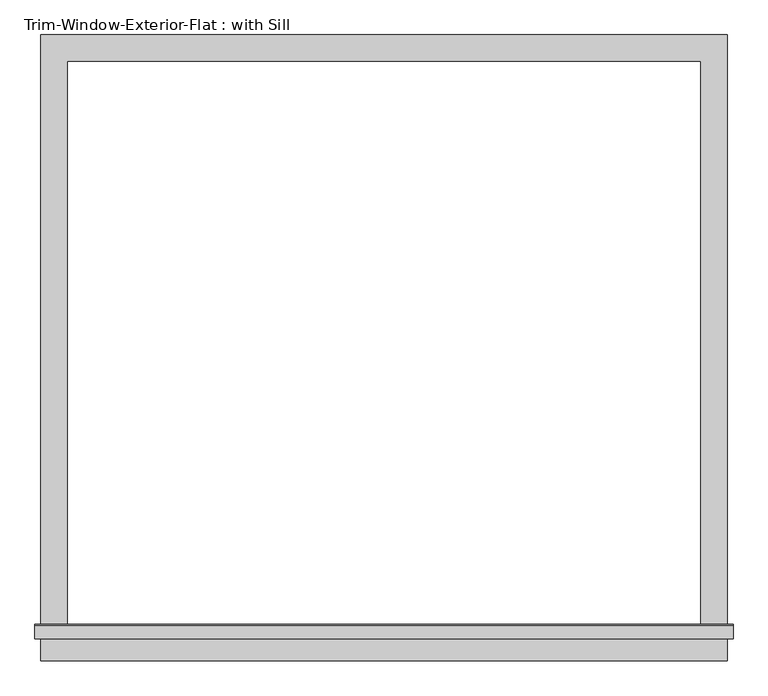
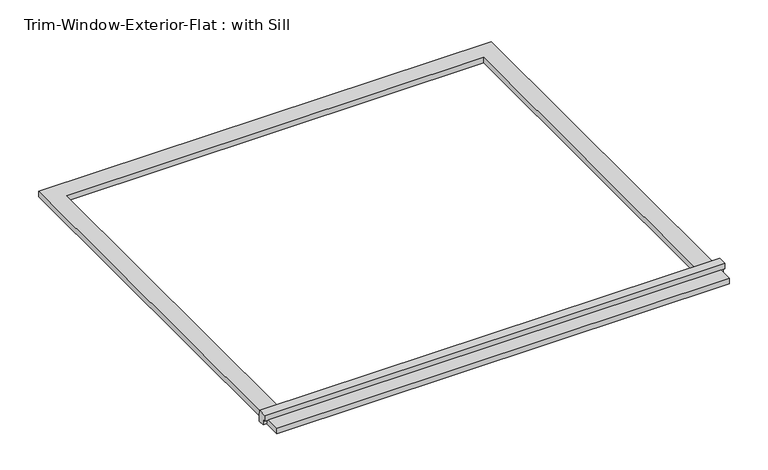
"""IFC4 building model written with IfcOpenShell, lengths in millimetres: proxy geometry, Trim-Window-Exterior-Flat : with Sill."""

from ifc_helpers import new_model, si_unit, frame, origin, origin_with_axes, place, context, project, spatial, polyline, outline, extrude, source, transform, mapped, element, save


def trim_window_exterior_flat_with_sill_5276bcf3(model_context):
    return source(origin(), model_context, "Body", "SweptSolid", [
        extrude(outline(polyline([(742.95, -1241.3823709), (742.95, -1298.5323709), (-742.95, -1298.5323709), (-742.95, -1241.3823709), (742.95, -1241.3823709)])), origin_with_axes(), (0.0, 0.0, 1.0), 19.05),
        extrude(outline(polyline([(-1250.95, 38.1), (-1221.6580645, 38.1), (-1219.2, 19.05), (-1219.2, 0.0), (-1241.3823709, 0.0), (-1241.3823709, 19.05), (-1250.95, 19.05), (-1250.95, 38.1)])), frame((-755.65, 0.0, 0.0), z_axis=(1.0, 0.0, 0.0), x_axis=(0.0, 1.0, 0.0)), (0.0, 0.0, 1.0), 1511.3),
        extrude(outline(polyline([(-742.95, 57.15), (742.95, 57.15), (742.95, -1219.2), (685.8, -1219.2), (685.8, 0.0), (-685.8, 0.0), (-685.8, -1219.2), (-742.95, -1219.2), (-742.95, 57.15)])), origin_with_axes(), (0.0, 0.0, 1.0), 19.05),
    ])


if __name__ == "__main__":
    model = new_model("IFC4")
    model_context = context("Model", 3, world=origin())
    ifc_project = project(units=[si_unit("LENGTHUNIT", "METRE", prefix="MILLI")], contexts=[model_context])
    site = spatial("IfcSite", under=ifc_project)
    building = spatial("IfcBuilding", under=site)
    placement = place(None, origin())
    trim_window_exterior_flat_with_sill_shape = trim_window_exterior_flat_with_sill_5276bcf3(model_context)
    element("IfcBuildingElementProxy", 1, Name="Trim-Window-Exterior-Flat : with Sill", ObjectType="Trim-Window-Exterior-Flat : with Sill", at=placement, inside=building, context=model_context, shape_type="MappedRepresentation", body=[
        mapped(trim_window_exterior_flat_with_sill_shape, transform((0.0, 0.0, 0.0), x_axis=(1.0, 0.0, 0.0), y_axis=(0.0, 1.0, 0.0), z_axis=(0.0, 0.0, 1.0))),
    ])
    save(model, "model.ifc")

# Revit data of these elements
# Type "Trim-Window-Exterior-Flat : with Sill"
#   Trim Width = 0' - 2 1/4"
#   Trim Thickness_Picture Frame = 0' - 1 1/4"
#   Trim Thickness_with Sill = 0' - 0 3/4"
#   Sill Thickness = 0' - 1 1/4"
#   Opening Width [instance default] = 2' - 0"
#   Opening Height [instance default] = 3' - 0"
#   Default Elevation = 4' - 0"
#   Sill = yes
#   Picture Frame = no
#   Trim Material [instance default] = none
# Element 1 (IfcBuildingElementProxy, "Trim-Window-Exterior-Flat : with Sill")
#   Opening Width = 4' - 6"
#   Opening Height = 4' - 0"
#   Trim Material = Clad - White
#   Materials on its faces: "Clad - White"
# Materials
#   "Clad - White": class "Wood", colour RGB 242 242 238, transparency 0, Cost = 0
